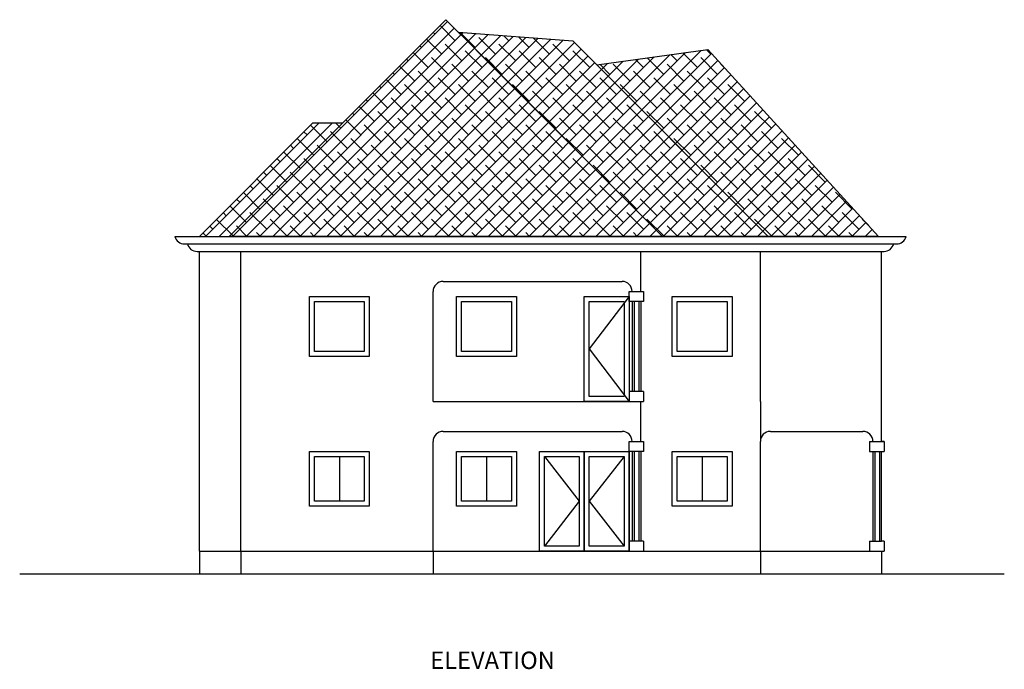
# Model space of a CAD drawing. Units: millimetres. Extents: x -857 to 54106, y -13666 to 13947.
# Tile 1 of 41: x -857 to 18850, y -13666 to -669. Entities that reach past the tile are written whole.
import ezdxf

# ---------------------------------------------------------------- set-up
doc = ezdxf.new("R2010")
doc.units = ezdxf.units.MM
for name, color, linetype, lineweight in [('A-ANNO-TEXT', 7, 'Continuous', 25), ('A-ELEV', 7, 'Continuous', 25), ('A-ELEV-PATT', 252, 'Continuous', 13)]:
    doc.layers.add(name, color=color, linetype=linetype, lineweight=lineweight)
doc.styles.get("Standard").update_dxf_attribs({"font": 'arial.ttf'})

msp = doc.modelspace()

# ---------------------------------------------------------------- hatches: boundary and pattern name
at = {"layer": 'A-ELEV-PATT'}
h = msp.add_hatch(dxfattribs=at)
h.set_pattern_fill('ANSI38', color=256, scale=60)
h.set_pattern_definition([(45, (-22719.68, -12808.97), (-134.7038, 134.7038), []), (135, (-22719.68, -12808.97), (-404.1115, 134.7038), [476.25, -285.75])])
h.paths.add_polyline_path([(8628.956, -1623.699), (7925.248, -919.991), (7674.129, -668.872), (3337.593, -5005.408), (12010.665, -5005.408)])
h.paths.add_polyline_path([(5602.593, -2740.408), (5003.867, -2740.408), (2738.867, -5005.408), (3337.593, -5005.408)])
h.paths.add_polyline_path([(10213.161, -1094.018), (7925.248, -919.991), (8628.956, -1623.699), (12010.665, -5005.408), (14124.551, -5005.408)])
h.paths.add_polyline_path([(12914.787, -1265.62), (10692.796, -1573.653), (14124.551, -5005.408), (16334.892, -5005.408)])

# ---------------------------------------------------------------- linework, layer by layer
at = {"layer": 'A-ELEV'}
for p, q in [((2248.631, -5005.408), (16885.913, -5005.408)), ((2442.28, -5155.408), (16692.264, -5155.408)), ((2692.28, -5305.408), (16442.264, -5305.408)), ((2742.28, -8305.408), (2742.28, -5305.408)), ((3567.28, -8305.408), (3567.28, -5305.408)), ((11572.675, -6105.408), (11572.675, -5305.408)), ((13967.28, -8305.408), (13967.28, -5305.408)), ((16392.264, -8305.408), (16392.264, -5305.408)), ((7617.28, -5905.408), (11199.781, -5905.408)), ((7417.28, -8305.408), (7417.28, -6105.408)), ((11343.636, -6105.408), (11627.524, -6105.408)), ((11343.636, -6305.408), (11343.636, -6105.408)), ((11627.524, -6105.408), (11627.524, -6305.408)), ((11343.585, -6205.408), (10543.585, -7255.408)), ((11627.524, -6305.408), (11343.636, -6305.408)), ((11399.781, -6305.408), (11399.781, -8105.408)), ((11439.781, -6305.408), (11439.781, -8105.408)), ((11532.675, -6305.408), (11532.675, -8105.408)), ((11572.675, -6305.408), (11572.675, -8105.408)), ((10543.585, -7255.408), (11343.585, -8305.408)), ((11343.636, -8105.408), (11343.636, -8305.408)), ((11627.524, -8105.408), (11343.636, -8105.408)), ((11627.524, -8105.408), (11627.524, -8305.408)), ((2742.28, -11305.408), (2742.28, -8305.408)), ((3567.28, -11305.408), (3567.28, -8305.408)), ((7417.28, -8305.408), (11627.524, -8305.408)), ((11572.624, -9105.408), (11572.624, -8305.408)), ((13967.28, -8305.408), (13967.28, -9105.408)), ((16392.264, -9105.408), (16392.264, -8305.408)), ((7617.28, -8905.408), (11199.73, -8905.408)), ((14167.28, -8905.408), (16020.041, -8905.408)), ((7417.28, -11305.408), (7417.28, -9105.408)), ((11343.585, -11305.408), (11343.585, -9105.408)), ((11343.585, -9105.408), (11627.473, -9105.408)), ((11627.473, -9105.408), (11627.473, -9305.408)), ((13967.28, -11305.408), (13967.28, -9105.408)), ((16155.07, -9105.408), (16392.264, -9105.408)), ((16155.07, -9105.408), (16155.07, -9305.408)), ((16163.896, -9105.408), (16447.783, -9105.408)), ((16447.783, -9105.408), (16392.264, -9105.408)), ((16447.783, -9105.408), (16447.783, -9305.408)), ((5540.719, -9405.408), (5540.719, -10305.408)), ((8486.254, -9405.408), (8486.254, -10305.408)), ((9643.585, -9405.408), (10343.167, -10305.408)), ((11243.585, -9405.408), (10543.167, -10305.408)), ((11627.473, -9305.408), (11343.585, -9305.408)), ((11399.73, -9305.408), (11399.73, -11105.408)), ((11439.73, -9305.408), (11439.73, -11105.408)), ((11532.624, -9305.408), (11532.624, -11105.408)), ((11572.624, -9305.408), (11572.624, -11105.408)), ((12200.793, -9305.408), (13400.793, -9305.408)), ((12800.793, -9405.408), (12800.793, -10305.408)), ((16155.07, -9305.408), (16392.264, -9305.408)), ((16220.041, -9305.408), (16220.041, -11105.408)), ((16260.041, -9305.408), (16260.041, -11105.408)), ((16352.934, -9305.408), (16352.934, -11105.408)), ((16392.264, -11105.408), (16392.264, -9305.408)), ((16392.264, -9305.408), (16447.783, -9305.408)), ((10343.167, -10305.408), (9643.585, -11205.408)), ((10543.167, -10305.408), (11243.585, -11205.408)), ((11343.585, -11105.408), (11343.585, -11305.408)), ((11627.473, -11105.408), (11343.585, -11105.408)), ((11627.473, -11105.408), (11627.473, -11305.408)), ((16155.07, -11105.408), (16155.07, -11305.408)), ((16155.07, -11105.408), (16392.264, -11105.408)), ((16447.783, -11105.408), (16392.264, -11105.408)), ((16447.783, -11105.408), (16447.783, -11305.408)), ((2742.28, -11305.408), (16392.264, -11305.408)), ((2742.28, -11305.408), (2742.28, -11755.408)), ((3567.28, -11305.408), (3567.28, -11755.408)), ((7417.28, -11305.408), (7417.28, -11755.408)), ((13967.28, -11305.408), (13967.28, -11755.408)), ((16392.264, -11305.408), (16392.264, -11755.408)), ((16392.264, -11305.408), (16447.783, -11305.408)), ((-857.311, -11755.408), (18850.136, -11755.408))]:
    msp.add_line(p, q, dxfattribs=at)
for points in [[(8305.442, -1300.184), (12011.159, -5005.902), (3337.593, -5005.408), (7674.129, -668.872)], [(10213.161, -1094.018), (14125.045, -5005.902), (12011.159, -5005.902), (8628.956, -1623.699), (7925.248, -919.991)], [(12914.787, -1265.62), (16335.344, -5005.902), (14125.045, -5005.902), (10692.796, -1573.653)], [(5003.867, -2740.408), (2738.867, -5005.408), (3337.593, -5005.408), (5602.593, -2740.408)], [(4940.719, -6205.408), (6140.719, -6205.408), (6140.719, -7405.408), (4940.719, -7405.408)], [(5040.719, -6305.408), (6040.719, -6305.408), (6040.719, -7305.408), (5040.719, -7305.408)], [(7886.254, -6205.408), (9086.254, -6205.408), (9086.254, -7405.408), (7886.254, -7405.408)], [(7986.254, -6305.408), (8986.254, -6305.408), (8986.254, -7305.408), (7986.254, -7305.408)], [(10443.585, -6205.408), (11343.585, -6205.408), (11343.585, -8305.408), (10443.585, -8305.408)], [(10543.585, -6305.408), (11243.585, -6305.408), (11243.585, -8205.408), (10543.585, -8205.408)], [(12200.793, -6205.408), (13400.793, -6205.408), (13400.793, -7405.408), (12200.793, -7405.408)], [(12300.793, -6305.408), (13300.793, -6305.408), (13300.793, -7305.408), (12300.793, -7305.408)], [(4940.719, -9305.408), (6140.719, -9305.408), (6140.719, -10405.408), (4940.719, -10405.408)], [(5040.719, -9405.408), (6040.719, -9405.408), (6040.719, -10305.408), (5040.719, -10305.408)], [(7886.254, -9305.408), (9086.254, -9305.408), (9086.254, -10405.408), (7886.254, -10405.408)], [(7986.254, -9405.408), (8986.254, -9405.408), (8986.254, -10305.408), (7986.254, -10305.408)], [(9543.585, -9305.408), (11343.585, -9305.408), (11343.585, -11305.408), (9543.585, -11305.408)], [(9543.585, -9305.408), (10443.167, -9305.408), (10443.167, -11305.408), (9543.585, -11305.408)], [(9643.585, -9405.408), (10343.167, -9405.408), (10343.167, -11205.408), (9643.585, -11205.408)], [(10443.167, -9305.408), (11343.585, -9305.408), (11343.585, -11305.408), (10443.167, -11305.408)], [(10543.167, -9405.408), (11243.585, -9405.408), (11243.585, -11205.408), (10543.167, -11205.408)], [(12200.793, -9305.408), (13400.793, -9305.408), (13400.793, -10405.408), (12200.793, -10405.408)], [(12300.793, -9405.408), (13300.793, -9405.408), (13300.793, -10305.408), (12300.793, -10305.408)]]:
    msp.add_lwpolyline(points, close=True, dxfattribs=at)
for centre, start, end in [((2442.28, -4955.408), 194.4775122, 270), ((16692.264, -4955.408), 270, 345.5224878), ((2692.28, -5105.408), 194.4775122, 270), ((16442.264, -5105.408), 270, 345.5224878), ((7617.28, -6105.408), 90, 180), ((11199.781, -6105.408), 0, 90), ((7617.28, -9105.408), 90, 180), ((11199.73, -9105.408), 0, 90), ((14167.28, -9105.408), 90, 180), ((16020.041, -9105.408), 0, 90)]:
    msp.add_arc(centre, 200, start, end, dxfattribs=at)

# ---------------------------------------------------------------- texts
at = {"layer": 'A-ANNO-TEXT', "insert": (7359.46, -13312.4), "char_height": 347.60543, "attachment_point": 1}
msp.add_mtext_dynamic_manual_height_columns('\\pxt0;ELEVATION', width=5900.0263, gutter_width=43450.679, heights=[5996.136], dxfattribs=at)

doc.saveas('drawing.dxf')
